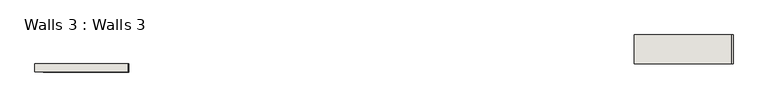
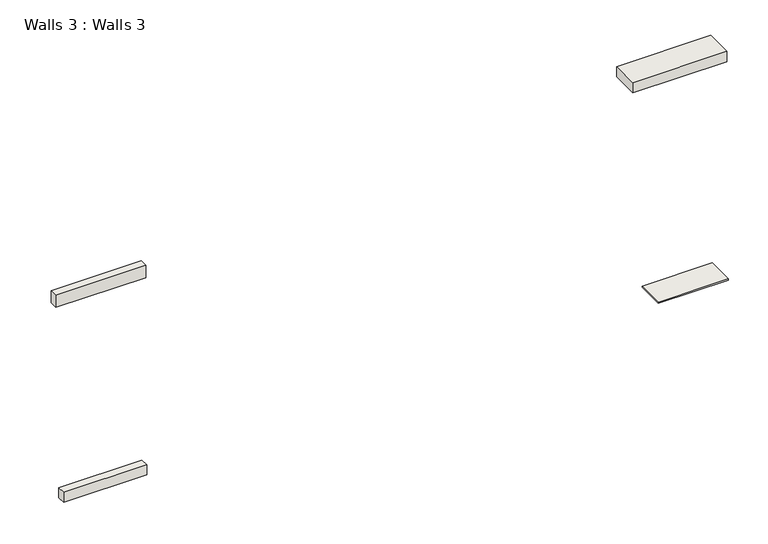
"""IFC4 building model written with IfcOpenShell, lengths in millimetres: wall geometry, Walls 3 : Walls 3."""

from ifc_helpers import new_model, si_unit, frame, origin, place, context, project, spatial, polyline, outline, extrude, source, transform, mapped, element, save


def walls_3_walls_3_d3df9a77(model_context):
    return source(origin(), model_context, "Body", "SweptSolid", [
        extrude(outline(polyline([(7230.4570664, -8799.4475106), (4309.98018, -8799.4475106), (4309.98018, -7932.8965627), (7230.4570664, -7932.8965627), (7230.4570664, -8799.4475106)])), frame((0.0, 0.0, 10785.288467), z_axis=(0.0, 0.0, 1.0), x_axis=(1.0, 0.0, 0.0)), (0.0, 0.0, 1.0), 336.2969849),
        extrude(outline(polyline([(7282.1796825, -8799.4475106), (5100.38018, -8799.4475106), (5100.38018, -7932.8965627), (7282.1796825, -7932.8965627), (7282.1796825, -8799.4475106)])), frame((0.0, 0.0, 3602.8433591), z_axis=(0.0, 0.0, 1.0), x_axis=(1.0, 0.0, 0.0)), (0.0, 0.0, 1.0), 36.7270077),
        extrude(outline(polyline([(-10942.4641624, -9049.4475106), (-13742.4641624, -9049.4475106), (-13742.4641624, -8799.4475106), (-10942.4641624, -8799.4475106), (-10942.4641624, -9049.4475106)])), frame((0.0, 0.0, 10215.8117107), z_axis=(0.0, 0.0, 1.0), x_axis=(1.0, 0.0, 0.0)), (0.0, 0.0, 1.0), 400.0),
        extrude(outline(polyline([(-10921.7453782, -9049.4475106), (-13497.0559029, -9049.4475106), (-13497.0559029, -8799.4475106), (-10921.7453782, -8799.4475106), (-10921.7453782, -9049.4475106)])), frame((0.0, 0.0, 3735.7955216), z_axis=(0.0, 0.0, 1.0), x_axis=(1.0, 0.0, 0.0)), (0.0, 0.0, 1.0), 327.8943742),
    ])


if __name__ == "__main__":
    model = new_model("IFC4")
    model_context = context("Model", 3, world=origin())
    ifc_project = project(units=[si_unit("LENGTHUNIT", "METRE", prefix="MILLI")], contexts=[model_context])
    site = spatial("IfcSite", under=ifc_project)
    building = spatial("IfcBuilding", under=site)
    placement = place(None, origin())
    walls_3_walls_3_shape = walls_3_walls_3_d3df9a77(model_context)
    element("IfcWall", 1, ObjectType="Walls 3 : Walls 3", at=placement, inside=building, context=model_context, shape_type="MappedRepresentation", body=[
        mapped(walls_3_walls_3_shape, transform((0.0, 0.0, 0.0), x_axis=(1.0, 0.0, 0.0), y_axis=(0.0, 1.0, 0.0), z_axis=(0.0, 0.0, 1.0))),
    ])
    save(model, "model.ifc")

# Revit data of these elements
# Element 1 (IfcWall, "Walls 3 : Walls 3")
#   Materials on its faces: "Default Wall"
# Materials
#   "Default Wall": colour RGB 80 80 80, transparency 0
